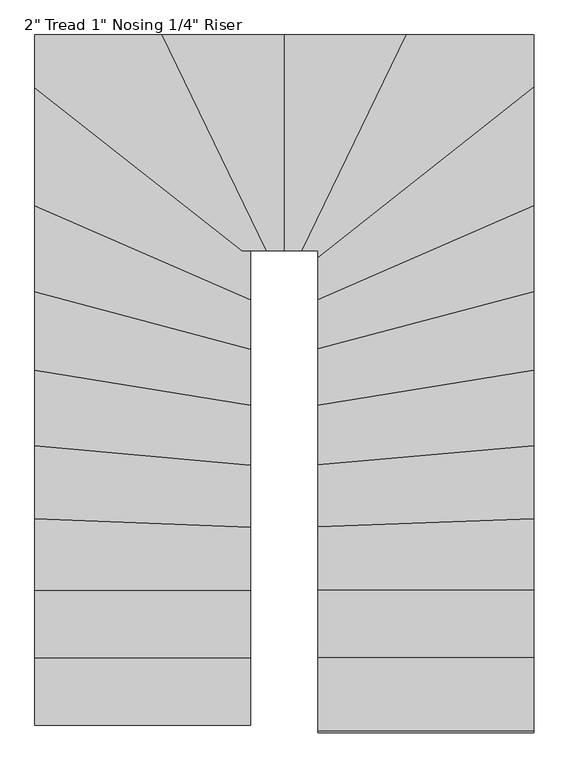
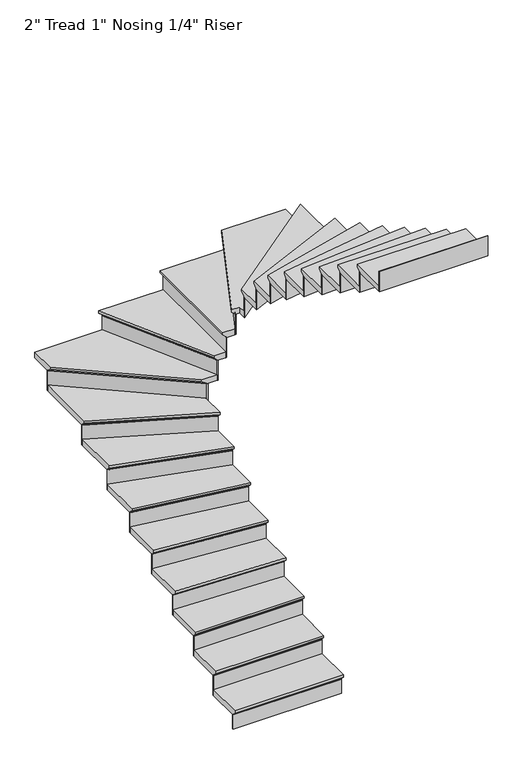
"""IFC4 building model written with IfcOpenShell, lengths in millimetres: stair flight geometry."""

from ifc_helpers import new_model, si_unit, origin, place, context, project, spatial, faceted_brep, source, transform, mapped, element, save


def stair_flight_2169dd6b(model_context):
    return source(origin(), model_context, "Body", "Brep", [
        faceted_brep([(-5047.1987704, -4554.2130548, 44046.3214286), (-5047.1987704, -4554.2130548, 44065.3714286), (-5940.8822214, -4554.2130548, 44065.3714286), (-5940.8822214, -4554.2130548, 44046.3214286), (-5047.1987704, -4528.8130548, 44020.9214286), (-5940.8822214, -4528.8130548, 44020.9214286), (-5047.1987704, -4249.4130548, 44065.3714286), (-5940.8822214, -4249.4130548, 44065.3714286), (-5940.8822214, -4528.8130548, 44014.5714286), (-5940.8822214, -4249.4130548, 44014.5714286), (-5047.1987704, -4249.4130548, 44014.5714286), (-5047.1987704, -4528.8130548, 44014.5714286)], [[[0, 1, 2, 3]], [[4, 0, 3, 5]], [[2, 1, 6, 7]], [[8, 9, 10, 11]], [[2, 7, 9, 8, 5, 3]], [[8, 11, 4, 5]], [[6, 1, 0, 4, 11, 10]], [[7, 6, 10, 9]]]),
        faceted_brep([(-5047.1987704, -4528.8130548, 44014.5714286), (-5047.1987704, -4528.8130548, 43891.2), (-5047.1987704, -4522.4630548, 43891.2), (-5047.1987704, -4522.4630548, 44014.5714286), (-5940.8822214, -4528.8130548, 44014.5714286), (-5940.8822214, -4522.4630548, 44014.5714286), (-5940.8822214, -4522.4630548, 43891.2), (-5940.8822214, -4528.8130548, 43891.2)], [[[0, 1, 2, 3]], [[4, 5, 6, 7]], [[1, 0, 4, 7]], [[2, 1, 7, 6]], [[3, 2, 6, 5]], [[0, 3, 5, 4]]]),
        faceted_brep([(-5047.1987704, -4249.4130548, 44188.7428571), (-5047.1987704, -4249.4130548, 44014.5714286), (-5047.1987704, -4243.0630548, 44014.5714286), (-5047.1987704, -4243.0630548, 44188.7428571), (-5940.8822214, -4249.4130548, 44188.7428571), (-5940.8822214, -4243.0630548, 44188.7428571), (-5940.8822214, -4243.0630548, 44014.5714286), (-5940.8822214, -4249.4130548, 44014.5714286)], [[[0, 1, 2, 3]], [[4, 5, 6, 7]], [[1, 0, 4, 7]], [[2, 1, 7, 6]], [[3, 2, 6, 5]], [[0, 3, 5, 4]]]),
        faceted_brep([(-5940.8822214, -4274.8130548, 44239.5428571), (-5047.1987704, -4274.8130548, 44239.5428571), (-5047.1987704, -3970.0130548, 44239.5428571), (-5940.8822214, -3970.0130548, 44239.5428571), (-5940.8822214, -4249.4130548, 44188.7428571), (-5940.8822214, -3970.0130548, 44188.7428571), (-5047.1987704, -3970.0130548, 44188.7428571), (-5047.1987704, -4249.4130548, 44188.7428571), (-5940.8822214, -4249.4130548, 44195.0928571), (-5940.8822214, -4274.8130548, 44220.4928571), (-5047.1987704, -4249.4130548, 44195.0928571), (-5047.1987704, -4274.8130548, 44220.4928571)], [[[0, 1, 2, 3]], [[4, 5, 6, 7]], [[0, 3, 5, 4, 8, 9]], [[4, 7, 10, 8]], [[2, 1, 11, 10, 7, 6]], [[3, 2, 6, 5]], [[11, 1, 0, 9]], [[10, 11, 9, 8]]]),
        faceted_brep([(-5047.1987704, -3970.0130548, 44362.9142857), (-5047.1987704, -3970.0130548, 44188.7428571), (-5047.1987704, -3963.6630548, 44188.7428571), (-5047.1987704, -3963.6630548, 44362.9142857), (-5940.8822214, -3970.0130548, 44362.9142857), (-5940.8822214, -3963.6630548, 44362.9142857), (-5940.8822214, -3963.6630548, 44188.7428571), (-5940.8822214, -3970.0130548, 44188.7428571)], [[[0, 1, 2, 3]], [[4, 5, 6, 7]], [[1, 0, 4, 7]], [[2, 1, 7, 6]], [[3, 2, 6, 5]], [[0, 3, 5, 4]]]),
        faceted_brep([(-5940.8822214, -3995.4130548, 44413.7142857), (-5047.1987704, -3995.4130548, 44413.7142857), (-5047.1987704, -3707.9036879, 44413.7142857), (-5940.8822214, -3673.2843203, 44413.7142857), (-5940.8822214, -3970.0130548, 44362.9142857), (-5940.8822214, -3673.2843203, 44362.9142857), (-5047.1987704, -3707.9036879, 44362.9142857), (-5047.1987704, -3970.0130548, 44362.9142857), (-5940.8822214, -3970.0130548, 44369.2642857), (-5940.8822214, -3995.4130548, 44394.6642857), (-5047.1987704, -3970.0130548, 44369.2642857), (-5047.1987704, -3995.4130548, 44394.6642857)], [[[0, 1, 2, 3]], [[4, 5, 6, 7]], [[0, 3, 5, 4, 8, 9]], [[4, 7, 10, 8]], [[2, 1, 11, 10, 7, 6]], [[3, 2, 6, 5]], [[11, 1, 0, 9]], [[10, 11, 9, 8]]]),
        faceted_brep([(-5047.1987704, -3707.9036879, 44537.0857143), (-5047.1987704, -3707.9036879, 44362.9142857), (-5047.1987704, -3701.5489252, 44362.9142857), (-5047.1987704, -3701.5489252, 44537.0857143), (-5940.8822214, -3673.2843203, 44537.0857143), (-5940.8822214, -3666.9295576, 44537.0857143), (-5940.8822214, -3666.9295576, 44362.9142857), (-5940.8822214, -3673.2843203, 44362.9142857)], [[[0, 1, 2, 3]], [[4, 5, 6, 7]], [[1, 0, 4, 7]], [[2, 1, 7, 6]], [[3, 2, 6, 5]], [[0, 3, 5, 4]]]),
        faceted_brep([(-5940.8822214, -3698.703371, 44587.8857143), (-5047.1987704, -3733.3227386, 44587.8857143), (-5047.1987704, -3451.3234819, 44587.8857143), (-5940.8822214, -3370.89733, 44587.8857143), (-5940.8822214, -3673.2843203, 44537.0857143), (-5940.8822214, -3370.89733, 44537.0857143), (-5047.1987704, -3451.3234819, 44537.0857143), (-5047.1987704, -3707.9036879, 44537.0857143), (-5940.8822214, -3673.2843203, 44543.4357143), (-5940.8822214, -3698.703371, 44568.8357143), (-5047.1987704, -3707.9036879, 44543.4357143), (-5047.1987704, -3733.3227386, 44568.8357143)], [[[0, 1, 2, 3]], [[4, 5, 6, 7]], [[0, 3, 5, 4, 8, 9]], [[4, 7, 10, 8]], [[2, 1, 11, 10, 7, 6]], [[3, 2, 6, 5]], [[11, 1, 0, 9]], [[10, 11, 9, 8]]]),
        faceted_brep([(-5047.1987704, -3451.3234819, 44711.2571429), (-5047.1987704, -3451.3234819, 44537.0857143), (-5047.1987704, -3444.9478197, 44537.0857143), (-5047.1987704, -3444.9478197, 44711.2571429), (-5940.8822214, -3370.89733, 44711.2571429), (-5940.8822214, -3364.5216678, 44711.2571429), (-5940.8822214, -3364.5216678, 44537.0857143), (-5940.8822214, -3370.89733, 44537.0857143)], [[[0, 1, 2, 3]], [[4, 5, 6, 7]], [[1, 0, 4, 7]], [[2, 1, 7, 6]], [[3, 2, 6, 5]], [[0, 3, 5, 4]]]),
        faceted_brep([(-5940.8822214, -3396.3999789, 44762.0571429), (-5047.1987704, -3476.8261308, 44762.0571429), (-5047.1987704, -3203.4301079, 44762.0571429), (-5940.8822214, -3059.5417727, 44762.0571429), (-5940.8822214, -3370.89733, 44711.2571429), (-5940.8822214, -3059.5417727, 44711.2571429), (-5047.1987704, -3203.4301079, 44711.2571429), (-5047.1987704, -3451.3234819, 44711.2571429), (-5940.8822214, -3370.89733, 44717.6071429), (-5940.8822214, -3396.3999789, 44743.0071429), (-5047.1987704, -3451.3234819, 44717.6071429), (-5047.1987704, -3476.8261308, 44743.0071429)], [[[0, 1, 2, 3]], [[4, 5, 6, 7]], [[0, 3, 5, 4, 8, 9]], [[4, 7, 10, 8]], [[2, 1, 11, 10, 7, 6]], [[3, 2, 6, 5]], [[11, 1, 0, 9]], [[10, 11, 9, 8]]]),
        faceted_brep([(-5047.1987704, -3203.4301079, 44885.4285714), (-5047.1987704, -3203.4301079, 44711.2571429), (-5047.1987704, -3196.9983292, 44711.2571429), (-5047.1987704, -3196.9983292, 44885.4285714), (-5940.8822214, -3059.5417727, 44885.4285714), (-5940.8822214, -3053.109994, 44885.4285714), (-5940.8822214, -3053.109994, 44711.2571429), (-5940.8822214, -3059.5417727, 44711.2571429)], [[[0, 1, 2, 3]], [[4, 5, 6, 7]], [[1, 0, 4, 7]], [[2, 1, 7, 6]], [[3, 2, 6, 5]], [[0, 3, 5, 4]]]),
        faceted_brep([(-5940.8822214, -3085.2688872, 44936.2285714), (-5047.1987704, -3229.1572224, 44936.2285714), (-5047.1987704, -2970.3553609, 44936.2285714), (-5940.8822214, -2732.7052783, 44936.2285714), (-5940.8822214, -3059.5417727, 44885.4285714), (-5940.8822214, -2732.7052783, 44885.4285714), (-5047.1987704, -2970.3553609, 44885.4285714), (-5047.1987704, -3203.4301079, 44885.4285714), (-5940.8822214, -3059.5417727, 44891.7785714), (-5940.8822214, -3085.2688872, 44917.1785714), (-5047.1987704, -3203.4301079, 44891.7785714), (-5047.1987704, -3229.1572224, 44917.1785714)], [[[0, 1, 2, 3]], [[4, 5, 6, 7]], [[0, 3, 5, 4, 8, 9]], [[4, 7, 10, 8]], [[2, 1, 11, 10, 7, 6]], [[3, 2, 6, 5]], [[11, 1, 0, 9]], [[10, 11, 9, 8]]]),
        faceted_brep([(-5047.1987704, -2970.3553609, 45059.6), (-5047.1987704, -2970.3553609, 44885.4285714), (-5047.1987704, -2963.7846771, 44885.4285714), (-5047.1987704, -2963.7846771, 45059.6), (-5940.8822214, -2732.7052783, 45059.6), (-5940.8822214, -2726.1345945, 45059.6), (-5940.8822214, -2726.1345945, 44885.4285714), (-5940.8822214, -2732.7052783, 44885.4285714)], [[[0, 1, 2, 3]], [[4, 5, 6, 7]], [[1, 0, 4, 7]], [[2, 1, 7, 6]], [[3, 2, 6, 5]], [[0, 3, 5, 4]]]),
        faceted_brep([(-5940.8822214, -2758.9880136, 45110.4), (-5047.1987704, -2996.6380961, 45110.4), (-5047.1987704, -2765.8050203, 45110.4), (-5940.8822214, -2375.5896532, 45110.4), (-5940.8822214, -2732.7052783, 45059.6), (-5940.8822214, -2375.5896532, 45059.6), (-5047.1987704, -2765.8050203, 45059.6), (-5047.1987704, -2970.3553609, 45059.6), (-5940.8822214, -2732.7052783, 45065.95), (-5940.8822214, -2758.9880136, 45091.35), (-5047.1987704, -2970.3553609, 45065.95), (-5047.1987704, -2996.6380961, 45091.35)], [[[0, 1, 2, 3]], [[4, 5, 6, 7]], [[0, 3, 5, 4, 8, 9]], [[4, 7, 10, 8]], [[2, 1, 11, 10, 7, 6]], [[3, 2, 6, 5]], [[11, 1, 0, 9]], [[10, 11, 9, 8]]]),
        faceted_brep([(-5047.1987704, -2765.8050203, 45233.7714286), (-5047.1987704, -2765.8050203, 45059.6), (-5047.1987704, -2758.8760908, 45059.6), (-5047.1987704, -2758.8760908, 45233.7714286), (-5940.8822214, -2375.5896532, 45233.7714286), (-5940.8822214, -2368.6607237, 45233.7714286), (-5940.8822214, -2368.6607237, 45059.6), (-5940.8822214, -2375.5896532, 45059.6)], [[[0, 1, 2, 3]], [[4, 5, 6, 7]], [[1, 0, 4, 7]], [[2, 1, 7, 6]], [[3, 2, 6, 5]], [[0, 3, 5, 4]]]),
        faceted_brep([(-5940.8822214, -2403.3053713, 45284.5714286), (-5047.1987704, -2793.5207384, 45284.5714286), (-5047.1987704, -2590.8424524, 45284.5714286), (-5040.8038639, -2590.8424524, 45284.5714286), (-5940.8822214, -1882.1944717, 45284.5714286), (-5940.8822214, -2375.5896532, 45233.7714286), (-5940.8822214, -1882.1944717, 45233.7714286), (-5040.8038639, -2590.8424524, 45233.7714286), (-5047.1987704, -2590.8424524, 45233.7714286), (-5047.1987704, -2765.8050203, 45233.7714286), (-5940.8822214, -2375.5896532, 45240.1214286), (-5940.8822214, -2403.3053713, 45265.5214286), (-5047.1987704, -2765.8050203, 45240.1214286), (-5047.1987704, -2793.5207384, 45265.5214286)], [[[0, 1, 2, 3, 4]], [[5, 6, 7, 8, 9]], [[0, 4, 6, 5, 10, 11]], [[5, 9, 12, 10]], [[2, 1, 13, 12, 9, 8]], [[4, 3, 7, 6]], [[13, 1, 0, 11]], [[12, 13, 11, 10]], [[3, 2, 8, 7]]]),
        faceted_brep([(-5040.8038639, -2590.8424524, 45407.9428571), (-5040.8038639, -2590.8424524, 45233.7714286), (-5030.5387554, -2590.8424524, 45233.7714286), (-5030.5387554, -2590.8424524, 45407.9428571), (-5940.8822214, -1882.1944717, 45407.9428571), (-5940.8822214, -1874.1125661, 45407.9428571), (-5940.8822214, -1874.1125661, 45233.7714286), (-5940.8822214, -1882.1944717, 45233.7714286)], [[[0, 1, 2, 3]], [[4, 5, 6, 7]], [[1, 0, 4, 7]], [[2, 1, 7, 6]], [[3, 2, 6, 5]], [[0, 3, 5, 4]]]),
        faceted_brep([(-5384.6489457, -1697.1590014, 45458.7428571), (-5940.8822214, -1697.1590014, 45458.7428571), (-5940.8822214, -1914.5220945, 45458.7428571), (-5081.8642978, -2590.8424524, 45458.7428571), (-4952.3566185, -2590.8424524, 45458.7428571), (-5940.8822214, -1697.1590014, 45407.9428571), (-5384.6489457, -1697.1590014, 45407.9428571), (-4952.3566185, -2590.8424524, 45407.9428571), (-5040.8038639, -2590.8424524, 45407.9428571), (-5940.8822214, -1882.1944717, 45407.9428571), (-5940.8822214, -1882.1944717, 45414.2928571), (-5940.8822214, -1914.5220945, 45439.6928571), (-5040.8038639, -2590.8424524, 45414.2928571), (-5081.8642978, -2590.8424524, 45439.6928571)], [[[0, 1, 2, 3, 4]], [[5, 6, 7, 8, 9]], [[1, 0, 6, 5]], [[2, 1, 5, 9, 10, 11]], [[9, 8, 12, 10]], [[4, 3, 13, 12, 8, 7]], [[0, 4, 7, 6]], [[13, 3, 2, 11]], [[12, 13, 11, 10]]]),
        faceted_brep([(-4952.3566185, -2590.8424524, 45582.1142857), (-4952.3566185, -2590.8424524, 45407.9428571), (-4945.3027294, -2590.8424524, 45407.9428571), (-4945.3027294, -2590.8424524, 45582.1142857), (-5384.6489457, -1697.1590014, 45582.1142857), (-5377.5950566, -1697.1590014, 45582.1142857), (-5377.5950566, -1697.1590014, 45407.9428571), (-5384.6489457, -1697.1590014, 45407.9428571)], [[[0, 1, 2, 3]], [[4, 5, 6, 7]], [[1, 0, 4, 7]], [[2, 1, 7, 6]], [[3, 2, 6, 5]], [[0, 3, 5, 4]]]),
        faceted_brep([(-5412.8645022, -1697.1590014, 45632.9142857), (-4980.5721749, -2590.8424524, 45632.9142857), (-4882.0987704, -2590.8424524, 45632.9142857), (-4882.0987706, -1697.1590014, 45632.9142857), (-5384.6489457, -1697.1590014, 45582.1142857), (-4882.0987706, -1697.1590014, 45582.1142857), (-4882.0987704, -2590.8424524, 45582.1142857), (-4952.3566185, -2590.8424524, 45582.1142857), (-5384.6489457, -1697.1590014, 45588.4642857), (-5412.8645022, -1697.1590014, 45613.8642857), (-4952.3566185, -2590.8424524, 45588.4642857), (-4980.5721749, -2590.8424524, 45613.8642857)], [[[0, 1, 2, 3]], [[4, 5, 6, 7]], [[0, 3, 5, 4, 8, 9]], [[4, 7, 10, 8]], [[3, 2, 6, 5]], [[11, 1, 0, 9]], [[10, 11, 9, 8]], [[2, 1, 11, 10, 7, 6]]]),
        faceted_brep([(-4882.0987704, -2590.8424524, 45756.2857143), (-4882.0987704, -2590.8424524, 45582.1142857), (-4875.7487704, -2590.8424524, 45582.1142857), (-4875.7487704, -2590.8424524, 45756.2857143), (-4882.0987706, -1697.1590014, 45756.2857143), (-4875.7487706, -1697.1590014, 45756.2857143), (-4875.7487706, -1697.1590014, 45582.1142857), (-4882.0987706, -1697.1590014, 45582.1142857)], [[[0, 1, 2, 3]], [[4, 5, 6, 7]], [[1, 0, 4, 7]], [[2, 1, 7, 6]], [[3, 2, 6, 5]], [[0, 3, 5, 4]]]),
        faceted_brep([(-4907.4987706, -1697.1590014, 45807.0857143), (-4907.4987704, -2590.8424524, 45807.0857143), (-4806.2098095, -2590.8424524, 45807.0857143), (-4373.9174828, -1697.1590014, 45807.0857143), (-4882.0987706, -1697.1590014, 45756.2857143), (-4373.9174828, -1697.1590014, 45756.2857143), (-4806.2098095, -2590.8424524, 45756.2857143), (-4882.0987704, -2590.8424524, 45756.2857143), (-4882.0987706, -1697.1590014, 45762.6357143), (-4907.4987706, -1697.1590014, 45788.0357143), (-4882.0987704, -2590.8424524, 45762.6357143), (-4907.4987704, -2590.8424524, 45788.0357143)], [[[0, 1, 2, 3]], [[4, 5, 6, 7]], [[0, 3, 5, 4, 8, 9]], [[4, 7, 10, 8]], [[2, 1, 11, 10, 7, 6]], [[3, 2, 6, 5]], [[11, 1, 0, 9]], [[10, 11, 9, 8]]]),
        faceted_brep([(-4806.2098095, -2590.8424524, 45930.4571429), (-4806.2098095, -2590.8424524, 45756.2857143), (-4799.1559204, -2590.8424524, 45756.2857143), (-4799.1559204, -2590.8424524, 45930.4571429), (-4373.9174828, -1697.1590014, 45930.4571429), (-4366.8635937, -1697.1590014, 45930.4571429), (-4366.8635937, -1697.1590014, 45756.2857143), (-4373.9174828, -1697.1590014, 45756.2857143)], [[[0, 1, 2, 3]], [[4, 5, 6, 7]], [[1, 0, 4, 7]], [[2, 1, 7, 6]], [[3, 2, 6, 5]], [[0, 3, 5, 4]]]),
        faceted_brep([(-3874.1153195, -1946.8497166, 45981.2571429), (-3874.1153195, -1697.1590014, 45981.2571429), (-4402.1330392, -1697.1590014, 45981.2571429), (-4834.4253659, -2590.8424524, 45981.2571429), (-4767.7987704, -2590.8424524, 45981.2571429), (-4767.7987704, -2650.4628721, 45981.2571429), (-3874.1153195, -1697.1590014, 45930.4571429), (-3874.1153195, -1946.8497166, 45930.4571429), (-4767.7987704, -2650.4628721, 45930.4571429), (-4767.7987704, -2590.8424524, 45930.4571429), (-4806.2098095, -2590.8424524, 45930.4571429), (-4373.9174828, -1697.1590014, 45930.4571429), (-4806.2098095, -2590.8424524, 45936.8071429), (-4373.9174828, -1697.1590014, 45936.8071429), (-4834.4253659, -2590.8424524, 45962.2071429), (-4402.1330392, -1697.1590014, 45962.2071429)], [[[0, 1, 2, 3, 4, 5]], [[6, 7, 8, 9, 10, 11]], [[1, 0, 7, 6]], [[11, 10, 12, 13]], [[4, 3, 14, 12, 10, 9]], [[5, 4, 9, 8]], [[0, 5, 8, 7]], [[14, 3, 2, 15]], [[12, 14, 15, 13]], [[2, 1, 6, 11, 13, 15]]]),
        faceted_brep([(-4767.7987704, -2650.4628721, 46104.6285714), (-4767.7987704, -2650.4628721, 45930.4571429), (-4767.7987704, -2658.5447778, 45930.4571429), (-4767.7987704, -2658.5447778, 46104.6285714), (-3874.1153195, -1946.8497166, 46104.6285714), (-3874.1153195, -1954.9316222, 46104.6285714), (-3874.1153195, -1954.9316222, 45930.4571429), (-3874.1153195, -1946.8497166, 45930.4571429)], [[[0, 1, 2, 3]], [[4, 5, 6, 7]], [[1, 0, 4, 7]], [[2, 1, 7, 6]], [[3, 2, 6, 5]], [[0, 3, 5, 4]]]),
        faceted_brep([(-3874.1153195, -1914.5220938, 46155.4285714), (-4767.7987704, -2618.1352494, 46155.4285714), (-4767.7987704, -2821.2364563, 46155.4285714), (-3874.1153195, -2431.0210889, 46155.4285714), (-3874.1153195, -1946.8497166, 46104.6285714), (-3874.1153195, -2431.0210889, 46104.6285714), (-4767.7987704, -2821.2364563, 46104.6285714), (-4767.7987704, -2650.4628721, 46104.6285714), (-3874.1153195, -1946.8497166, 46110.9785714), (-3874.1153195, -1914.5220938, 46136.3785714), (-4767.7987704, -2650.4628721, 46110.9785714), (-4767.7987704, -2618.1352494, 46136.3785714)], [[[0, 1, 2, 3]], [[4, 5, 6, 7]], [[0, 3, 5, 4, 8, 9]], [[4, 7, 10, 8]], [[2, 1, 11, 10, 7, 6]], [[3, 2, 6, 5]], [[11, 1, 0, 9]], [[10, 11, 9, 8]]]),
        faceted_brep([(-4767.7987704, -2821.2364563, 46278.8), (-4767.7987704, -2821.2364563, 46104.6285714), (-4767.7987704, -2828.1653858, 46104.6285714), (-4767.7987704, -2828.1653858, 46278.8), (-3874.1153195, -2431.0210889, 46278.8), (-3874.1153195, -2437.9500185, 46278.8), (-3874.1153195, -2437.9500185, 46104.6285714), (-3874.1153195, -2431.0210889, 46104.6285714)], [[[0, 1, 2, 3]], [[4, 5, 6, 7]], [[1, 0, 4, 7]], [[2, 1, 7, 6]], [[3, 2, 6, 5]], [[0, 3, 5, 4]]]),
        faceted_brep([(-3874.1153195, -2403.3053709, 46329.6), (-4767.7987704, -2793.5207382, 46329.6), (-4767.7987704, -3022.9208311, 46329.6), (-3874.1153195, -2785.2707484, 46329.6), (-3874.1153195, -2431.0210889, 46278.8), (-3874.1153195, -2785.2707484, 46278.8), (-4767.7987704, -3022.9208311, 46278.8), (-4767.7987704, -2821.2364563, 46278.8), (-3874.1153195, -2431.0210889, 46285.15), (-3874.1153195, -2403.3053709, 46310.55), (-4767.7987704, -2821.2364563, 46285.15), (-4767.7987704, -2793.5207382, 46310.55)], [[[0, 1, 2, 3]], [[4, 5, 6, 7]], [[0, 3, 5, 4, 8, 9]], [[4, 7, 10, 8]], [[2, 1, 11, 10, 7, 6]], [[3, 2, 6, 5]], [[11, 1, 0, 9]], [[10, 11, 9, 8]]]),
        faceted_brep([(-4767.7987704, -3022.9208311, 46452.9714286), (-4767.7987704, -3022.9208311, 46278.8), (-4767.7987704, -3029.4915149, 46278.8), (-4767.7987704, -3029.4915149, 46452.9714286), (-3874.1153195, -2785.2707484, 46452.9714286), (-3874.1153195, -2791.8414322, 46452.9714286), (-3874.1153195, -2791.8414322, 46278.8), (-3874.1153195, -2785.2707484, 46278.8)], [[[0, 1, 2, 3]], [[4, 5, 6, 7]], [[1, 0, 4, 7]], [[2, 1, 7, 6]], [[3, 2, 6, 5]], [[0, 3, 5, 4]]]),
        faceted_brep([(-3874.1153195, -2758.9880132, 46503.7714286), (-4767.7987704, -2996.6380959, 46503.7714286), (-4767.7987704, -3254.8843368, 46503.7714286), (-3874.1153195, -3110.9960015, 46503.7714286), (-3874.1153195, -2785.2707484, 46452.9714286), (-3874.1153195, -3110.9960015, 46452.9714286), (-4767.7987704, -3254.8843368, 46452.9714286), (-4767.7987704, -3022.9208311, 46452.9714286), (-3874.1153195, -2785.2707484, 46459.3214286), (-3874.1153195, -2758.9880132, 46484.7214286), (-4767.7987704, -3022.9208311, 46459.3214286), (-4767.7987704, -2996.6380959, 46484.7214286)], [[[0, 1, 2, 3]], [[4, 5, 6, 7]], [[0, 3, 5, 4, 8, 9]], [[4, 7, 10, 8]], [[2, 1, 11, 10, 7, 6]], [[3, 2, 6, 5]], [[11, 1, 0, 9]], [[10, 11, 9, 8]]]),
        faceted_brep([(-4767.7987704, -3254.8843368, 46627.1428571), (-4767.7987704, -3254.8843368, 46452.9714286), (-4767.7987704, -3261.3161154, 46452.9714286), (-4767.7987704, -3261.3161154, 46627.1428571), (-3874.1153195, -3110.9960015, 46627.1428571), (-3874.1153195, -3117.4277801, 46627.1428571), (-3874.1153195, -3117.4277801, 46452.9714286), (-3874.1153195, -3110.9960015, 46452.9714286)], [[[0, 1, 2, 3]], [[4, 5, 6, 7]], [[1, 0, 4, 7]], [[2, 1, 7, 6]], [[3, 2, 6, 5]], [[0, 3, 5, 4]]]),
        faceted_brep([(-3874.1153195, -3085.2688869, 46677.9428571), (-4767.7987704, -3229.1572222, 46677.9428571), (-4767.7987704, -3502.3287795, 46677.9428571), (-3874.1153195, -3421.9026274, 46677.9428571), (-3874.1153195, -3110.9960015, 46627.1428571), (-3874.1153195, -3421.9026274, 46627.1428571), (-4767.7987704, -3502.3287795, 46627.1428571), (-4767.7987704, -3254.8843368, 46627.1428571), (-3874.1153195, -3110.9960015, 46633.4928571), (-3874.1153195, -3085.2688869, 46658.8928571), (-4767.7987704, -3254.8843368, 46633.4928571), (-4767.7987704, -3229.1572222, 46658.8928571)], [[[0, 1, 2, 3]], [[4, 5, 6, 7]], [[0, 3, 5, 4, 8, 9]], [[4, 7, 10, 8]], [[2, 1, 11, 10, 7, 6]], [[3, 2, 6, 5]], [[11, 1, 0, 9]], [[10, 11, 9, 8]]]),
        faceted_brep([(-4767.7987704, -3502.3287795, 46801.3142857), (-4767.7987704, -3502.3287795, 46627.1428571), (-4767.7987704, -3508.7044417, 46627.1428571), (-4767.7987704, -3508.7044417, 46801.3142857), (-3874.1153195, -3421.9026274, 46801.3142857), (-3874.1153195, -3428.2782897, 46801.3142857), (-3874.1153195, -3428.2782897, 46627.1428571), (-3874.1153195, -3421.9026274, 46627.1428571)], [[[0, 1, 2, 3]], [[4, 5, 6, 7]], [[1, 0, 4, 7]], [[2, 1, 7, 6]], [[3, 2, 6, 5]], [[0, 3, 5, 4]]]),
        faceted_brep([(-3874.1153195, -3396.3999786, 46852.1142857), (-4767.7987704, -3476.8261306, 46852.1142857), (-4767.7987704, -3758.7417891, 46852.1142857), (-3874.1153195, -3724.1224215, 46852.1142857), (-3874.1153195, -3421.9026274, 46801.3142857), (-3874.1153195, -3724.1224215, 46801.3142857), (-4767.7987704, -3758.7417891, 46801.3142857), (-4767.7987704, -3502.3287795, 46801.3142857), (-3874.1153195, -3421.9026274, 46807.6642857), (-3874.1153195, -3396.3999786, 46833.0642857), (-4767.7987704, -3502.3287795, 46807.6642857), (-4767.7987704, -3476.8261306, 46833.0642857)], [[[0, 1, 2, 3]], [[4, 5, 6, 7]], [[0, 3, 5, 4, 8, 9]], [[4, 7, 10, 8]], [[2, 1, 11, 10, 7, 6]], [[3, 2, 6, 5]], [[11, 1, 0, 9]], [[10, 11, 9, 8]]]),
        faceted_brep([(-4767.7987704, -3758.7417891, 46975.4857143), (-4767.7987704, -3758.7417891, 46801.3142857), (-4767.7987704, -3765.0965518, 46801.3142857), (-4767.7987704, -3765.0965518, 46975.4857143), (-3874.1153195, -3724.1224215, 46975.4857143), (-3874.1153195, -3730.4771842, 46975.4857143), (-3874.1153195, -3730.4771842, 46801.3142857), (-3874.1153195, -3724.1224215, 46801.3142857)], [[[0, 1, 2, 3]], [[4, 5, 6, 7]], [[1, 0, 4, 7]], [[2, 1, 7, 6]], [[3, 2, 6, 5]], [[0, 3, 5, 4]]]),
        faceted_brep([(-3874.1153195, -3698.7033708, 47026.2857143), (-4767.7987704, -3733.3227384, 47026.2857143), (-4767.7987704, -4020.8130546, 47026.2857143), (-3874.1153195, -4020.8130546, 47026.2857143), (-3874.1153195, -3724.1224215, 46975.4857143), (-3874.1153195, -4020.8130546, 46975.4857143), (-4767.7987704, -4020.8130546, 46975.4857143), (-4767.7987704, -3758.7417891, 46975.4857143), (-3874.1153195, -3724.1224215, 46981.8357143), (-3874.1153195, -3698.7033708, 47007.2357143), (-4767.7987704, -3758.7417891, 46981.8357143), (-4767.7987704, -3733.3227384, 47007.2357143)], [[[0, 1, 2, 3]], [[4, 5, 6, 7]], [[0, 3, 5, 4, 8, 9]], [[4, 7, 10, 8]], [[2, 1, 11, 10, 7, 6]], [[3, 2, 6, 5]], [[11, 1, 0, 9]], [[10, 11, 9, 8]]]),
        faceted_brep([(-4767.7987704, -4020.8130546, 47149.6571429), (-4767.7987704, -4020.8130546, 46975.4857143), (-4767.7987704, -4027.1630546, 46975.4857143), (-4767.7987704, -4027.1630546, 47149.6571429), (-3874.1153195, -4020.8130546, 47149.6571429), (-3874.1153195, -4027.1630546, 47149.6571429), (-3874.1153195, -4027.1630546, 46975.4857143), (-3874.1153195, -4020.8130546, 46975.4857143)], [[[0, 1, 2, 3]], [[4, 5, 6, 7]], [[1, 0, 4, 7]], [[2, 1, 7, 6]], [[3, 2, 6, 5]], [[0, 3, 5, 4]]]),
        faceted_brep([(-3874.1153195, -3995.4130546, 47200.4571429), (-4767.7987704, -3995.4130546, 47200.4571429), (-4767.7987704, -4300.2130546, 47200.4571429), (-3874.1153195, -4300.2130546, 47200.4571429), (-3874.1153195, -4020.8130546, 47149.6571429), (-3874.1153195, -4300.2130546, 47149.6571429), (-4767.7987704, -4300.2130546, 47149.6571429), (-4767.7987704, -4020.8130546, 47149.6571429), (-3874.1153195, -4020.8130546, 47156.0071429), (-3874.1153195, -3995.4130546, 47181.4071429), (-4767.7987704, -4020.8130546, 47156.0071429), (-4767.7987704, -3995.4130546, 47181.4071429)], [[[0, 1, 2, 3]], [[4, 5, 6, 7]], [[0, 3, 5, 4, 8, 9]], [[4, 7, 10, 8]], [[2, 1, 11, 10, 7, 6]], [[3, 2, 6, 5]], [[11, 1, 0, 9]], [[10, 11, 9, 8]]]),
        faceted_brep([(-4767.7987704, -4300.2130546, 47323.8285714), (-4767.7987704, -4300.2130546, 47149.6571429), (-4767.7987704, -4306.5630546, 47149.6571429), (-4767.7987704, -4306.5630546, 47323.8285714), (-3874.1153195, -4300.2130546, 47323.8285714), (-3874.1153195, -4306.5630546, 47323.8285714), (-3874.1153195, -4306.5630546, 47149.6571429), (-3874.1153195, -4300.2130546, 47149.6571429)], [[[0, 1, 2, 3]], [[4, 5, 6, 7]], [[1, 0, 4, 7]], [[2, 1, 7, 6]], [[3, 2, 6, 5]], [[0, 3, 5, 4]]]),
        faceted_brep([(-4767.7987704, -4579.6130546, 47498.0), (-4767.7987704, -4579.6130546, 47323.8285714), (-4767.7987704, -4585.9630546, 47323.8285714), (-4767.7987704, -4585.9630546, 47498.0), (-3874.1153195, -4579.6130546, 47498.0), (-3874.1153195, -4585.9630546, 47498.0), (-3874.1153195, -4585.9630546, 47323.8285714), (-3874.1153195, -4579.6130546, 47323.8285714)], [[[0, 1, 2, 3]], [[4, 5, 6, 7]], [[1, 0, 4, 7]], [[2, 1, 7, 6]], [[3, 2, 6, 5]], [[0, 3, 5, 4]]]),
        faceted_brep([(-3874.1153195, -4274.8130546, 47374.6285714), (-4767.7987704, -4274.8130546, 47374.6285714), (-4767.7987704, -4579.6130546, 47374.6285714), (-3874.1153195, -4579.6130546, 47374.6285714), (-3874.1153195, -4300.2130546, 47323.8285714), (-3874.1153195, -4579.6130546, 47323.8285714), (-4767.7987704, -4579.6130546, 47323.8285714), (-4767.7987704, -4300.2130546, 47323.8285714), (-3874.1153195, -4300.2130546, 47330.1785714), (-3874.1153195, -4274.8130546, 47355.5785714), (-4767.7987704, -4300.2130546, 47330.1785714), (-4767.7987704, -4274.8130546, 47355.5785714)], [[[0, 1, 2, 3]], [[4, 5, 6, 7]], [[0, 3, 5, 4, 8, 9]], [[4, 7, 10, 8]], [[2, 1, 11, 10, 7, 6]], [[3, 2, 6, 5]], [[11, 1, 0, 9]], [[10, 11, 9, 8]]]),
    ])


if __name__ == "__main__":
    model = new_model("IFC4")
    model_context = context("Model", 3, world=origin())
    ifc_project = project(units=[si_unit("LENGTHUNIT", "METRE", prefix="MILLI")], contexts=[model_context])
    site = spatial("IfcSite", under=ifc_project)
    building = spatial("IfcBuilding", under=site)
    placement = place(None, origin())
    stair_flight_shape = stair_flight_2169dd6b(model_context)
    element("IfcStairFlight", 1, ObjectType="2\" Tread 1\" Nosing 1/4\" Riser", at=placement, inside=building, context=model_context, shape_type="MappedRepresentation", body=[
        mapped(stair_flight_shape, transform((0.0, 0.0, 0.0), x_axis=(1.0, 0.0, 0.0), y_axis=(0.0, 1.0, 0.0), z_axis=(0.0, 0.0, 1.0))),
    ])
    save(model, "model.ifc")

# Revit data of these elements
# Element 1 (IfcStairFlight, "2\" Tread 1\" Nosing 1/4\" Riser")
#   Materials on its faces: "Tile, Porcelain, 4in"
# Materials
#   "Tile, Porcelain, 4in": class "Generic", colour RGB 89 87 158, transparency 0, Description = "Porcelain tile, 4\", white", Cost = 0
